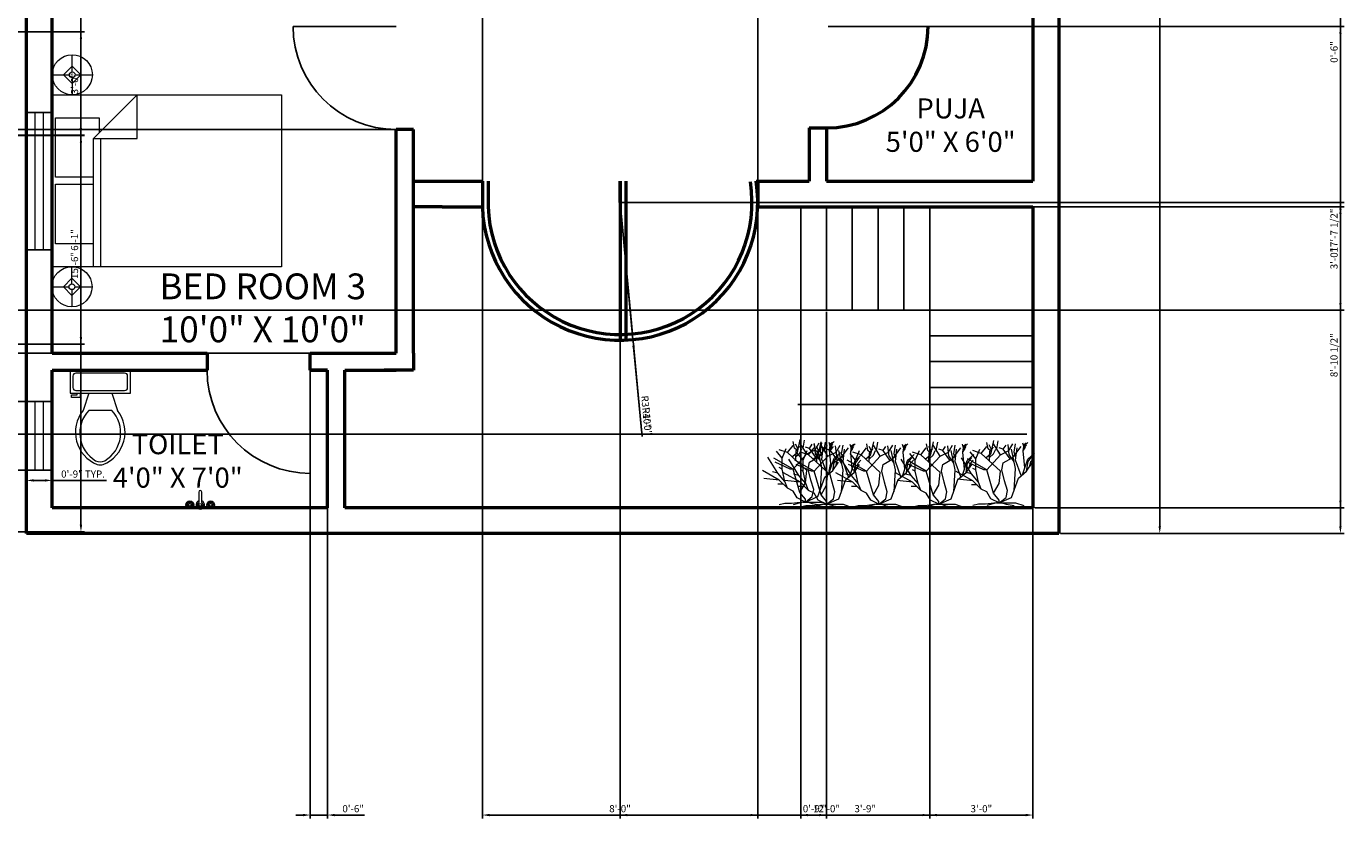
# Model space of a CAD drawing. Units: inches. Extents: x 3688 to 4628, y 1593 to 2337.
# Tile 5 of 7: x 4168 to 4628, y 1596 to 1872. Entities that reach past the tile are written whole.
import ezdxf

# ---------------------------------------------------------------- set-up
doc = ezdxf.new("R2010")
doc.units = ezdxf.units.IN
for name, color, linetype, lineweight in [('A-ANNO-DIMS', 2, 'Continuous', 18), ('A-AREA-IDEN', 7, 'Continuous', 25), ('A-DOOR', 4, 'Continuous', 25), ('A-FLOR-FIXT', 8, 'Continuous', 18), ('A-FLOR-STRS', 3, 'Continuous', 25), ('A-FURN', 8, 'Continuous', 18), ('A-GLAZ', 4, 'Continuous', 25), ('A-WALL', 7, 'Continuous', 50), ('L-PLNT', 3, 'Continuous', 13)]:
    doc.layers.add(name, color=color, linetype=linetype, lineweight=lineweight)
doc.styles.get("Standard").update_dxf_attribs({"font": 'arial.ttf'})
doc.dimstyles.new('ISO-25', dxfattribs={"dimtxt": 2.5, "dimasz": 2.5, "dimexe": 1.25, "dimexo": 0.625, "dimtad": 1, "dimdec": 0, "dimlunit": 3, "dimtxsty": 'Standard', "dimcen": 2.5, "dimadec": 0, "dimazin": 0, "dimtfac": 1, "dimtdec": 0, "dimtmove": 0, "dimatfit": 3, "dimfxl": 1, "dimarcsym": 0})

# ---------------------------------------------------------------- blocks, each defined once
blk = doc.blocks.new('Toilet - top')
for p, q in [((9.5, -6), (9.5, -2)), ((-10, -8.5), (-8, -8.5)), ((-10, -9.5), (-10, -8.5)), ((-8, -8.5), (-8, -8)), ((-7, -8), (-7, -9.5)), ((-4, -8), (-6, -14)), ((4, -8), (6, -14)), ((-7, -9.5), (-10, -9.5)), ((4, -14), (-4, -14))]:
    blk.add_line(p, q)
blk.add_lwpolyline([(10.5, -8), (10.5, 0), (-10.5, 0), (-10.5, -8)], close=True)
for points in [[(-9.5, -2), (-9.5, -6)], [(8.5, -1), (-8.5, -1)], [(-8.5, -7), (8.5, -7)]]:
    blk.add_lwpolyline(points)
for centre, radius, start, end in [((-8.62, -1.88), 0.884, 81.8699, 188.1301), ((8.62, -1.88), 0.884, 351.8699, 98.1301), ((-8.62, -6.12), 0.884, 171.8699, 278.1301), ((8.62, -6.12), 0.884, 261.8699, 8.1301), ((3.52, -21.58), 12.17, 141.4691, 247.9714), ((4.2, -21.82), 11.33, 136.3677, 238.9468), ((-3.52, -21.58), 12.17, 292.0284, 38.5307), ((-4.2, -21.82), 11.33, 301.053, 43.6321), ((0, -27.88), 4, 245.7318, 294.2682), ((0, -29), 4, 254.8605, 285.1395)]:
    blk.add_arc(centre, radius, start, end)
blk = doc.blocks.new('Faucet - Bathroom top')
for p, q in [((-4.107, 0.125), (-4.375, 0.125)), ((-3.75, 0.4788), (-3.75, 0.75)), ((-3.5, 0.482), (-3.5, 0.75)), ((-3.1461, 0.125), (-2.875, 0.125)), ((3.143, 0.125), (2.875, 0.125)), ((3.5, 0.4788), (3.5, 0.75)), ((3.75, 0.482), (3.75, 0.75)), ((4.1039, 0.125), (4.375, 0.125)), ((-4.1039, -0.125), (-4.375, -0.125)), ((-3.75, -0.4821), (-3.75, -0.75)), ((-3.5, -0.4789), (-3.5, -0.75)), ((-3.143, -0.125), (-2.875, -0.125)), ((-0.5, -0.8639), (-0.5, -4.5)), ((0.5, -4.5), (0.5, -0.8631)), ((3.1461, -0.125), (2.875, -0.125)), ((3.5, -0.4821), (3.5, -0.75)), ((3.75, -0.4789), (3.75, -0.75)), ((4.107, -0.125), (4.375, -0.125))]:
    blk.add_line(p, q)
for centre, radius in [((-3.625, 0), 1.375), ((-4.625, 0), 0.2795), ((-3.625, 0), 0.5), ((-3.625, 1), 0.2795), ((-2.625, 0), 0.2795), ((0, 0), 0.5), ((3.625, 0), 1.375), ((2.625, 0), 0.2795), ((3.625, 0), 0.5), ((3.625, 1), 0.2795), ((4.625, 0), 0.2795), ((-3.625, -1), 0.2795), ((3.625, -1), 0.2795)]:
    blk.add_circle(centre, radius)
for centre, radius, start, end in [((-3.625, 0), 1, 105.2407, 164.2093), ((-3.625, 0), 1, 16.44125, 74.07887), ((0, 0), 1.5, 289.6514, 250.3603), ((0, 0), 1, 300.3431, 239.7554), ((3.625, 0), 1, 106.12, 164.0884), ((3.625, 0), 1, 16.23422, 73.90469), ((-3.625, 0), 1, 196.2342, 253.9047), ((-3.625, 0), 1, 286.12, 344.0884), ((0, -4.5), 0.5, 180, 0), ((3.625, 0), 1, 196.4413, 254.0789), ((3.625, 0), 1, 285.2407, 344.2093)]:
    blk.add_arc(centre, radius, start, end)
blk = doc.blocks.new('Bed - Queen')
for p, q in [((0, -80.00003), (0, 0)), ((0, 0), (59.99999, 0)), ((59.99999, 0), (59.99999, -80.00003)), ((7.99999, -1.2), (28.79998, -1.2)), ((7.99999, -14.4), (7.99999, -1.2)), ((28.79998, -1.2), (28.79998, -14.4)), ((31.19999, -1.2), (51.99999, -1.2)), ((31.19999, -14.4), (31.19999, -1.2)), ((51.99999, -1.2), (51.99999, -16.4)), ((0, -14.4), (44.8, -14.4)), ((44.8, -16.8), (0, -16.8)), ((59.99999, -29.6), (44.8, -14.4)), ((44.8, -14.4), (44.8, -29.6)), ((51.99999, -16.4), (46.79936, -16.4)), ((44.8, -29.6), (59.99999, -29.6)), ((59.99999, -80.00003), (0, -80.00003))]:
    blk.add_line(p, q)
blk = doc.blocks.new('Lamp - Table')
for p, q in [((0, 7), (0, 1)), ((-1, 0), (-7, 0)), ((0, 3), (-3, 0)), ((-3, 0), (0, -3)), ((3, 0), (0, 3)), ((0, -3), (3, 0)), ((1, 0), (7, 0)), ((0, -1), (0, -7))]:
    blk.add_line(p, q)
for radius in [7, 1]:
    blk.add_circle((0, 0), radius)
blk = doc.blocks.new('*U12')
for p, q in [((-16.8, 16.32), (-18.72, 18.72)), ((-14.88, 18.24), (-17.76, 19.2)), ((-16.8, 16.32), (-15.36, 19.68)), ((-14.88, 18.24), (-12.96, 20.64)), ((-12.471, 19.775), (-12.898, 22.044)), ((-11.677, 19.071), (-12.471, 19.775)), ((-11.28, 19.619), (-12.104, 21.184)), ((-12.043, 15.628), (-11.921, 18.836)), ((-11.921, 18.836), (-10.64, 20.401)), ((-11.433, 18.289), (-10.457, 22.749)), ((-10.579, 18.054), (-9.846, 19.697)), ((-8.16, 17.76), (-10.56, 21.6)), ((-9.48, 19.775), (-8.992, 22.592)), ((-7.2, 19.68), (-8.64, 20.16)), ((-8.16, 17.76), (-5.28, 19.2)), ((-7.2, 19.68), (-6.24, 21.12)), ((-4.8, 16.32), (-7.2, 19.68)), ((-5.086, 17.741), (-5.513, 21.34)), ((-5.28, 19.2), (-3.84, 21.6)), ((-2.88, 12.96), (-4.32, 19.68)), ((-3.84, 16.8), (-0.96, 20.64)), ((-3.377, 18.602), (-2.888, 21.575)), ((-2.766, 16.802), (-3.377, 18.602)), ((-2.88, 15.84), (-2.4, 20.16)), ((-0.508, 21.888), (-0.081, 20.558)), ((-0.203, 19.149), (0.102, 21.34)), ((0.346, 13.203), (-0.203, 19.149)), ((-0.142, 19.384), (0.59, 20.401)), ((-0.02, 20.01), (0.896, 21.105)), ((0.041, 20.714), (1.384, 22.044)), ((0.102, 21.34), (0.835, 21.888)), ((-18.24, 11.04), (-21.755, 16.655)), ((-12.96, 12.48), (-19.68, 16.32)), ((-13.92, 12.48), (-19.2, 14.88)), ((-16.8, 12.48), (-16.8, 16.32)), ((-8.16, 12), (-14.88, 18.24)), ((-13.325, 16.724), (-11.433, 18.289)), ((-12.96, 12.48), (-8.16, 17.76)), ((-11.982, 16.802), (-10.579, 18.054)), ((-7.68, 12.48), (-7.2, 14.88)), ((-7.2, 14.88), (-3.84, 16.8)), ((-3.377, 15.315), (-5.086, 17.819)), ((-0.96, 10.56), (-2.88, 15.84)), ((0.346, 13.203), (1.323, 16.254)), ((0.96, 12), (1.44, 15.36)), ((0.96, 12), (2.88, 14.88)), ((1.323, 16.254), (3.642, 18.289)), ((1.44, 15.36), (2.88, 17.28)), ((1.92, 13.44), (2.4, 15.36)), ((2.4, 15.36), (3.36, 16.32)), ((-17.76, 8.64), (-23.663, 11.961)), ((-17.76, 8.64), (-23.128, 9.222)), ((-18.24, 11.04), (-20.16, 11.52)), ((-15.84, 8.16), (-18.24, 11.04)), ((-16.8, 12.48), (-17.76, 12.96)), ((-15.84, 8.16), (-16.8, 12.48)), ((-12.96, 12.48), (-13.92, 12.48)), ((-10.56, 4.32), (-12.96, 12.48)), ((-8.64, 7.68), (-8.16, 12)), ((-6.72, 8.64), (-7.68, 12.48)), ((-4.32, 2.88), (-1.92, 9.6)), ((-3.36, 5.28), (-2.88, 12.96)), ((-1.92, 9.6), (0.96, 12)), ((-0.48, 10.8), (0.346, 13.203)), ((-16.32, 7.2), (-18.24, 7.2)), ((-14.88, 5.76), (-17.76, 8.64)), ((-14.88, 5.76), (-15.84, 8.16)), ((-12.96, 4.8), (-14.88, 5.76)), ((-11.52, 2.4), (-12.96, 4.8)), ((-10.56, 4.32), (-8.64, 7.68)), ((-5.76, 5.28), (-6.72, 8.64)), ((-6.24, 2.88), (-5.76, 5.28)), ((-15.84, 0.48), (-17.76, 0)), ((-13.44, 0.48), (-15.84, 0.48)), ((-9.6, 0.96), (-13.44, 0.48)), ((-9.6, 0.96), (-12.96, 0)), ((-8.64, 0.96), (-11.52, 2.4)), ((-8.64, 1.92), (-10.56, 4.32)), ((-9.6, 0.96), (-7.68, 0.96)), ((-8.64, 0.96), (-4.32, 2.88)), ((-8.64, 0.96), (-6.24, 2.88)), ((-8.64, 0.96), (-8.64, 1.92)), ((-8.64, 0.96), (-2.88, 0.96)), ((-7.68, 0.96), (-6.24, 0.48)), ((-6.24, 0.48), (-3.36, 0)), ((-2.88, 0.96), (0, 0))]:
    blk.add_line(p, q)
blk = doc.blocks.new('*D15')
at = {"layer": 'A-ANNO-DIMS', "color": 0, "lineweight": -2, "transparency": 16777216}
for p, q in [((4528.76, 2295.28), (4564.58, 2295.28)), ((4563.33, 2292.78), (4563.33, 1697.78)), ((4528.76, 1695.28), (4564.58, 1695.28))]:
    blk.add_line(p, q, dxfattribs=at)
at = {"layer": 'A-ANNO-DIMS', "color": 0, "transparency": 16777216}
for points in [[(4562.91, 2292.78), (4563.75, 2292.78), (4563.33, 2295.28)], [(4562.91, 1697.78), (4563.75, 1697.78), (4563.33, 1695.28)]]:
    blk.add_solid(points, dxfattribs=at)
at = {"layer": 'Defpoints', "color": 0, "transparency": 16777216}
for p in [(4528.13, 2295.28), (4528.13, 1695.28), (4563.33, 1695.28)]:
    blk.add_point(p, dxfattribs=at)
at = {"layer": 'A-ANNO-DIMS', "color": 0, "transparency": 16777216, "insert": (4561.43, 1995.28), "char_height": 2.5, "attachment_point": 5, "rotation": 90}
blk.add_mtext("50'", dxfattribs=at)
blk = doc.blocks.new('DOOR-900')
blk.add_line((0, 0), (0, 36))
blk.add_arc((0, 0), 36, 0, 90)
blk = doc.blocks.new('WIN-1200')
for p, q in [((0, 48), (0, 0)), ((9, 48), (0, 48)), ((9, 0), (9, 48)), ((0, 0), (9, 0))]:
    blk.add_line(p, q)
blk = doc.blocks.new('WIN-600')
for p, q in [((24, 9), (0, 9)), ((0, 9), (0, 0)), ((24, 0), (24, 9)), ((0, 0), (24, 0))]:
    blk.add_line(p, q)
blk = doc.blocks.new('*D25')
at = {"layer": 'A-ANNO-DIMS', "color": 0, "lineweight": -2, "transparency": 16777216}
for p, q in [((4167.51, 1741.42), (4163.28, 1741.42)), ((4164.53, 1738.92), (4164.53, 1719.92)), ((4167.51, 1717.42), (4163.28, 1717.42)), ((4164.53, 1717.42), (4164.53, 1662.98))]:
    blk.add_line(p, q, dxfattribs=at)
at = {"layer": 'A-ANNO-DIMS', "color": 0, "transparency": 16777216}
for points in [[(4164.12, 1738.92), (4164.95, 1738.92), (4164.53, 1741.42)], [(4164.12, 1719.92), (4164.95, 1719.92), (4164.53, 1717.42)]]:
    blk.add_solid(points, dxfattribs=at)
at = {"layer": 'Defpoints', "color": 0, "transparency": 16777216}
for p in [(4168.13, 1741.42), (4164.53, 1717.42), (4168.13, 1717.42)]:
    blk.add_point(p, dxfattribs=at)
at = {"layer": 'A-ANNO-DIMS', "color": 0, "transparency": 16777216, "insert": (4162.27, 1688.95), "char_height": 2.5, "attachment_point": 5, "rotation": 90}
blk.add_mtext('VENTILATOR V (600) 2\'-0" TYP.', dxfattribs=at)
blk = doc.blocks.new('*D26')
at = {"layer": 'A-ANNO-DIMS', "color": 0, "lineweight": -2, "transparency": 16777216}
for p, q in [((4168.13, 1716.8), (4168.13, 1712.57)), ((4177.13, 1716.8), (4177.13, 1712.57)), ((4170.63, 1713.82), (4174.63, 1713.82)), ((4177.13, 1713.82), (4196.12, 1713.82))]:
    blk.add_line(p, q, dxfattribs=at)
at = {"layer": 'A-ANNO-DIMS', "color": 0, "transparency": 16777216}
for points in [[(4170.63, 1714.24), (4170.63, 1713.41), (4168.13, 1713.82)], [(4174.63, 1714.24), (4174.63, 1713.41), (4177.13, 1713.82)]]:
    blk.add_solid(points, dxfattribs=at)
at = {"layer": 'Defpoints', "color": 0, "transparency": 16777216}
for p in [(4168.13, 1717.42), (4177.13, 1717.42), (4177.13, 1713.82)]:
    blk.add_point(p, dxfattribs=at)
at = {"layer": 'A-ANNO-DIMS', "color": 0, "transparency": 16777216, "insert": (4187.88, 1715.72), "char_height": 2.5, "attachment_point": 5}
blk.add_mtext('0\'-9" TYP.', dxfattribs=at)
blk = doc.blocks.new('*D61')
at = {"layer": 'A-ANNO-DIMS', "color": 0, "lineweight": -2, "transparency": 16777216}
for p, q in [((4090.25, 1881.84), (4188.4, 1881.84)), ((4187.15, 1879.34), (4187.15, 1698.33)), ((4090.03, 1695.83), (4188.4, 1695.83))]:
    blk.add_line(p, q, dxfattribs=at)
at = {"layer": 'A-ANNO-DIMS', "color": 0, "transparency": 16777216}
for points in [[(4186.74, 1879.34), (4187.57, 1879.34), (4187.15, 1881.84)], [(4186.74, 1698.33), (4187.57, 1698.33), (4187.15, 1695.83)]]:
    blk.add_solid(points, dxfattribs=at)
at = {"layer": 'Defpoints', "color": 0, "transparency": 16777216}
for p in [(4089.62, 1881.84), (4089.41, 1695.83), (4187.15, 1695.83)]:
    blk.add_point(p, dxfattribs=at)
at = {"layer": 'A-ANNO-DIMS', "color": 0, "transparency": 16777216, "insert": (4185.25, 1788.83), "char_height": 2.5, "attachment_point": 5, "rotation": 90}
blk.add_mtext('15\'-6"', dxfattribs=at)
blk = doc.blocks.new('*D78')
at = {"layer": 'A-ANNO-DIMS', "color": 0, "lineweight": -2, "transparency": 16777216}
for p, q in [((3973.25, 1870.32), (4188.4, 1870.32)), ((4187.15, 1867.82), (4187.15, 1836.82)), ((3973.25, 1834.32), (4188.4, 1834.32))]:
    blk.add_line(p, q, dxfattribs=at)
at = {"layer": 'A-ANNO-DIMS', "color": 0, "transparency": 16777216}
for points in [[(4186.74, 1867.82), (4187.57, 1867.82), (4187.15, 1870.32)], [(4186.74, 1836.82), (4187.57, 1836.82), (4187.15, 1834.32)]]:
    blk.add_solid(points, dxfattribs=at)
at = {"layer": 'Defpoints', "color": 0, "transparency": 16777216}
for p in [(3972.62, 1870.32), (3972.62, 1834.32), (4187.15, 1834.32)]:
    blk.add_point(p, dxfattribs=at)
at = {"layer": 'A-ANNO-DIMS', "color": 0, "transparency": 16777216, "insert": (4185.25, 1852.32), "char_height": 2.5, "attachment_point": 5, "rotation": 90}
blk.add_mtext('3\'-0"', dxfattribs=at)
blk = doc.blocks.new('*D79')
at = {"layer": 'A-ANNO-DIMS', "color": 0, "lineweight": -2, "transparency": 16777216}
for p, q in [((4044.44, 1834.15), (4188.4, 1834.15)), ((4187.15, 1831.65), (4187.15, 1763.82)), ((4045.25, 1761.32), (4188.4, 1761.32))]:
    blk.add_line(p, q, dxfattribs=at)
at = {"layer": 'A-ANNO-DIMS', "color": 0, "transparency": 16777216}
for points in [[(4186.74, 1831.65), (4187.57, 1831.65), (4187.15, 1834.15)], [(4186.74, 1763.82), (4187.57, 1763.82), (4187.15, 1761.32)]]:
    blk.add_solid(points, dxfattribs=at)
at = {"layer": 'Defpoints', "color": 0, "transparency": 16777216}
for p in [(4043.81, 1834.15), (4044.62, 1761.32), (4187.15, 1761.32)]:
    blk.add_point(p, dxfattribs=at)
at = {"layer": 'A-ANNO-DIMS', "color": 0, "transparency": 16777216, "insert": (4185.25, 1797.73), "char_height": 2.5, "attachment_point": 5, "rotation": 90}
blk.add_mtext('6\'-1"', dxfattribs=at)
blk = doc.blocks.new('*D88')
at = {"layer": 'A-ANNO-DIMS', "color": 0, "lineweight": -2, "transparency": 16777216}
for p, q in [((4528.76, 1906.79), (4627.58, 1906.79)), ((4626.33, 1904.29), (4626.33, 1697.78)), ((4528.76, 1695.28), (4627.58, 1695.28))]:
    blk.add_line(p, q, dxfattribs=at)
at = {"layer": 'A-ANNO-DIMS', "color": 0, "transparency": 16777216}
for points in [[(4625.91, 1904.29), (4626.74, 1904.29), (4626.33, 1906.79)], [(4625.91, 1697.78), (4626.74, 1697.78), (4626.33, 1695.28)]]:
    blk.add_solid(points, dxfattribs=at)
at = {"layer": 'Defpoints', "color": 0, "transparency": 16777216}
for p in [(4528.13, 1906.79), (4528.13, 1695.28), (4626.33, 1695.28)]:
    blk.add_point(p, dxfattribs=at)
at = {"layer": 'A-ANNO-DIMS', "color": 0, "transparency": 16777216, "insert": (4624.41, 1801.03), "char_height": 2.5, "attachment_point": 5, "rotation": 90}
blk.add_mtext('17\'-7 1/2"', dxfattribs=at)
blk = doc.blocks.new('*D100')
at = {"layer": 'A-ANNO-DIMS', "color": 0, "lineweight": -2, "transparency": 16777216}
for p, q in [((4327.13, 1883.66), (4327.13, 1595.79)), ((4423.13, 1883.66), (4423.13, 1595.79)), ((4329.63, 1597.04), (4420.63, 1597.04))]:
    blk.add_line(p, q, dxfattribs=at)
at = {"layer": 'A-ANNO-DIMS', "color": 0, "transparency": 16777216}
for points in [[(4329.63, 1597.45), (4329.63, 1596.62), (4327.13, 1597.04)], [(4420.63, 1597.45), (4420.63, 1596.62), (4423.13, 1597.04)]]:
    blk.add_solid(points, dxfattribs=at)
at = {"layer": 'Defpoints', "color": 0, "transparency": 16777216}
for p in [(4327.13, 1884.28), (4423.13, 1884.28), (4423.13, 1597.04)]:
    blk.add_point(p, dxfattribs=at)
at = {"layer": 'A-ANNO-DIMS', "color": 0, "transparency": 16777216, "insert": (4375.13, 1598.94), "char_height": 2.5, "attachment_point": 5}
blk.add_mtext('8\'-0"', dxfattribs=at)
blk = doc.blocks.new('*D101')
at = {"layer": 'A-ANNO-DIMS', "color": 0, "lineweight": -2, "transparency": 16777216}
for p, q in [((4056.49, 1886.78), (4056.49, 1889.28)), ((4296.51, 1884.28), (4055.24, 1884.28)), ((4056.49, 1884.28), (4056.49, 1878.28)), ((4296.51, 1878.28), (4055.24, 1878.28)), ((4056.49, 1875.78), (4056.49, 1865.39))]:
    blk.add_line(p, q, dxfattribs=at)
at = {"layer": 'A-ANNO-DIMS', "color": 0, "transparency": 16777216}
for points in [[(4056.07, 1886.78), (4056.9, 1886.78), (4056.49, 1884.28)], [(4056.07, 1875.78), (4056.9, 1875.78), (4056.49, 1878.28)]]:
    blk.add_solid(points, dxfattribs=at)
at = {"layer": 'Defpoints', "color": 0, "transparency": 16777216}
for p in [(4297.13, 1884.28), (4056.49, 1878.28), (4297.13, 1878.28)]:
    blk.add_point(p, dxfattribs=at)
at = {"layer": 'A-ANNO-DIMS', "color": 0, "transparency": 16777216, "insert": (4054.58, 1869.34), "char_height": 2.5, "attachment_point": 5, "rotation": 90}
blk.add_mtext('0\'-6"', dxfattribs=at)
blk = doc.blocks.new('*D102')
at = {"layer": 'A-ANNO-DIMS', "color": 0, "lineweight": -2, "transparency": 16777216}
for p, q in [((4296.51, 1836.28), (4055.24, 1836.28)), ((4056.49, 1833.78), (4056.49, 1760.78)), ((4296.51, 1758.28), (4055.24, 1758.28))]:
    blk.add_line(p, q, dxfattribs=at)
at = {"layer": 'A-ANNO-DIMS', "color": 0, "transparency": 16777216}
for points in [[(4056.07, 1833.78), (4056.9, 1833.78), (4056.49, 1836.28)], [(4056.07, 1760.78), (4056.9, 1760.78), (4056.49, 1758.28)]]:
    blk.add_solid(points, dxfattribs=at)
at = {"layer": 'Defpoints', "color": 0, "transparency": 16777216}
for p in [(4297.13, 1836.28), (4056.49, 1758.28), (4297.13, 1758.28)]:
    blk.add_point(p, dxfattribs=at)
at = {"layer": 'A-ANNO-DIMS', "color": 0, "transparency": 16777216, "insert": (4054.58, 1797.28), "char_height": 2.5, "attachment_point": 5, "rotation": 90}
blk.add_mtext('6\'-6"', dxfattribs=at)
blk = doc.blocks.new('*D103')
at = {"layer": 'A-ANNO-DIMS', "color": 0, "lineweight": -2, "transparency": 16777216}
for p, q in [((4626.33, 1880.78), (4626.33, 1883.28)), ((4447.76, 1878.28), (4627.58, 1878.28)), ((4626.33, 1878.28), (4626.33, 1872.28)), ((4447.76, 1872.28), (4627.58, 1872.28)), ((4626.33, 1869.78), (4626.33, 1859.39))]:
    blk.add_line(p, q, dxfattribs=at)
at = {"layer": 'A-ANNO-DIMS', "color": 0, "transparency": 16777216}
for points in [[(4625.91, 1880.78), (4626.74, 1880.78), (4626.33, 1878.28)], [(4625.91, 1869.78), (4626.74, 1869.78), (4626.33, 1872.28)]]:
    blk.add_solid(points, dxfattribs=at)
at = {"layer": 'Defpoints', "color": 0, "transparency": 16777216}
for p in [(4447.13, 1878.28), (4447.13, 1872.28), (4626.33, 1872.28)]:
    blk.add_point(p, dxfattribs=at)
at = {"layer": 'A-ANNO-DIMS', "color": 0, "transparency": 16777216, "insert": (4624.43, 1863.34), "char_height": 2.5, "attachment_point": 5, "rotation": 90}
blk.add_mtext('0\'-6"', dxfattribs=at)
blk = doc.blocks.new('*D104')
at = {"layer": 'A-ANNO-DIMS', "color": 0, "lineweight": -2, "transparency": 16777216}
for p, q in [((4267.13, 1751.66), (4267.13, 1595.79)), ((4273.13, 1751.66), (4273.13, 1595.79)), ((4264.63, 1597.04), (4262.13, 1597.04)), ((4267.13, 1597.04), (4273.13, 1597.04)), ((4275.63, 1597.04), (4286.03, 1597.04))]:
    blk.add_line(p, q, dxfattribs=at)
at = {"layer": 'A-ANNO-DIMS', "color": 0, "transparency": 16777216}
for points in [[(4264.63, 1597.45), (4264.63, 1596.62), (4267.13, 1597.04)], [(4275.63, 1597.45), (4275.63, 1596.62), (4273.13, 1597.04)]]:
    blk.add_solid(points, dxfattribs=at)
at = {"layer": 'Defpoints', "color": 0, "transparency": 16777216}
for p in [(4267.13, 1752.28), (4273.13, 1752.28), (4273.13, 1597.04)]:
    blk.add_point(p, dxfattribs=at)
at = {"layer": 'A-ANNO-DIMS', "color": 0, "transparency": 16777216, "insert": (4282.08, 1598.94), "char_height": 2.5, "attachment_point": 5}
blk.add_mtext('0\'-6"', dxfattribs=at)
blk = doc.blocks.new('*D105')
at = {"layer": 'A-ANNO-DIMS', "color": 0, "lineweight": -2, "transparency": 16777216}
for p, q in [((4375.76, 1810.76), (4627.58, 1810.76)), ((4626.33, 1808.26), (4626.33, 1706.78)), ((4519.76, 1704.28), (4627.58, 1704.28))]:
    blk.add_line(p, q, dxfattribs=at)
at = {"layer": 'A-ANNO-DIMS', "color": 0, "transparency": 16777216}
for points in [[(4625.91, 1808.26), (4626.74, 1808.26), (4626.33, 1810.76)], [(4625.91, 1706.78), (4626.74, 1706.78), (4626.33, 1704.28)]]:
    blk.add_solid(points, dxfattribs=at)
at = {"layer": 'Defpoints', "color": 0, "transparency": 16777216}
for p in [(4375.13, 1810.76), (4519.13, 1704.28), (4626.33, 1704.28)]:
    blk.add_point(p, dxfattribs=at)
at = {"layer": 'A-ANNO-DIMS', "color": 0, "transparency": 16777216, "insert": (4624.41, 1757.52), "char_height": 2.5, "attachment_point": 5, "rotation": 90}
blk.add_mtext('8\'-10 1/2"', dxfattribs=at)
blk = doc.blocks.new('*D106')
at = {"layer": 'A-ANNO-DIMS', "color": 0, "lineweight": -2, "transparency": 16777216}
for p, q in [((4375.13, 1810.13), (4375.13, 1595.79)), ((4519.13, 1808.66), (4519.13, 1595.79)), ((4377.63, 1597.04), (4516.63, 1597.04))]:
    blk.add_line(p, q, dxfattribs=at)
at = {"layer": 'A-ANNO-DIMS', "color": 0, "transparency": 16777216}
for points in [[(4377.63, 1597.45), (4377.63, 1596.62), (4375.13, 1597.04)], [(4516.63, 1597.45), (4516.63, 1596.62), (4519.13, 1597.04)]]:
    blk.add_solid(points, dxfattribs=at)
at = {"layer": 'Defpoints', "color": 0, "transparency": 16777216}
for p in [(4375.13, 1810.76), (4519.13, 1809.28), (4519.13, 1597.04)]:
    blk.add_point(p, dxfattribs=at)
at = {"layer": 'A-ANNO-DIMS', "color": 0, "transparency": 16777216, "insert": (4447.13, 1598.94), "char_height": 2.5, "attachment_point": 5}
blk.add_mtext('12\'-0"', dxfattribs=at)
blk = doc.blocks.new('*D107')
at = {"layer": 'A-ANNO-DIMS', "color": 0, "lineweight": -2, "transparency": 16777216}
for p, q in [((4438.13, 1808.66), (4438.13, 1595.79)), ((4483.13, 1808.66), (4483.13, 1595.79)), ((4440.63, 1597.04), (4480.63, 1597.04))]:
    blk.add_line(p, q, dxfattribs=at)
at = {"layer": 'A-ANNO-DIMS', "color": 0, "transparency": 16777216}
for points in [[(4440.63, 1597.45), (4440.63, 1596.62), (4438.13, 1597.04)], [(4480.63, 1597.45), (4480.63, 1596.62), (4483.13, 1597.04)]]:
    blk.add_solid(points, dxfattribs=at)
at = {"layer": 'Defpoints', "color": 0, "transparency": 16777216}
for p in [(4438.13, 1809.28), (4483.13, 1809.28), (4483.13, 1597.04)]:
    blk.add_point(p, dxfattribs=at)
at = {"layer": 'A-ANNO-DIMS', "color": 0, "transparency": 16777216, "insert": (4460.63, 1598.94), "char_height": 2.5, "attachment_point": 5}
blk.add_mtext('3\'-9"', dxfattribs=at)
blk = doc.blocks.new('*D108')
at = {"layer": 'A-ANNO-DIMS', "color": 0, "lineweight": -2, "transparency": 16777216}
for p, q in [((4483.13, 1808.66), (4483.13, 1595.79)), ((4519.13, 1808.66), (4519.13, 1595.79)), ((4485.63, 1597.04), (4516.63, 1597.04))]:
    blk.add_line(p, q, dxfattribs=at)
at = {"layer": 'A-ANNO-DIMS', "color": 0, "transparency": 16777216}
for points in [[(4485.63, 1597.45), (4485.63, 1596.62), (4483.13, 1597.04)], [(4516.63, 1597.45), (4516.63, 1596.62), (4519.13, 1597.04)]]:
    blk.add_solid(points, dxfattribs=at)
at = {"layer": 'Defpoints', "color": 0, "transparency": 16777216}
for p in [(4483.13, 1809.28), (4519.13, 1809.28), (4519.13, 1597.04)]:
    blk.add_point(p, dxfattribs=at)
at = {"layer": 'A-ANNO-DIMS', "color": 0, "transparency": 16777216, "insert": (4501.13, 1598.94), "char_height": 2.5, "attachment_point": 5}
blk.add_mtext('3\'-0"', dxfattribs=at)
blk = doc.blocks.new('*D109')
at = {"layer": 'A-ANNO-DIMS', "color": 0, "lineweight": -2, "transparency": 16777216}
for p, q in [((4438.13, 1772.66), (4438.13, 1595.79)), ((4447.13, 1772.66), (4447.13, 1595.79)), ((4440.63, 1597.04), (4444.63, 1597.04))]:
    blk.add_line(p, q, dxfattribs=at)
at = {"layer": 'A-ANNO-DIMS', "color": 0, "transparency": 16777216}
for points in [[(4440.63, 1597.45), (4440.63, 1596.62), (4438.13, 1597.04)], [(4444.63, 1597.45), (4444.63, 1596.62), (4447.13, 1597.04)]]:
    blk.add_solid(points, dxfattribs=at)
at = {"layer": 'Defpoints', "color": 0, "transparency": 16777216}
for p in [(4438.13, 1773.28), (4447.13, 1773.28), (4447.13, 1597.04)]:
    blk.add_point(p, dxfattribs=at)
at = {"layer": 'A-ANNO-DIMS', "color": 0, "transparency": 16777216, "insert": (4442.63, 1598.94), "char_height": 2.5, "attachment_point": 5}
blk.add_mtext('0\'-9"', dxfattribs=at)
blk = doc.blocks.new('*D110')
at = {"layer": 'A-ANNO-DIMS', "color": 0, "lineweight": -2, "transparency": 16777216}
for p, q in [((4438.76, 1809.28), (4627.58, 1809.28)), ((4626.33, 1806.78), (4626.33, 1775.78)), ((4438.76, 1773.28), (4627.58, 1773.28))]:
    blk.add_line(p, q, dxfattribs=at)
at = {"layer": 'A-ANNO-DIMS', "color": 0, "transparency": 16777216}
for points in [[(4625.91, 1806.78), (4626.74, 1806.78), (4626.33, 1809.28)], [(4625.91, 1775.78), (4626.74, 1775.78), (4626.33, 1773.28)]]:
    blk.add_solid(points, dxfattribs=at)
at = {"layer": 'Defpoints', "color": 0, "transparency": 16777216}
for p in [(4438.13, 1809.28), (4438.13, 1773.28), (4626.33, 1773.28)]:
    blk.add_point(p, dxfattribs=at)
at = {"layer": 'A-ANNO-DIMS', "color": 0, "transparency": 16777216, "insert": (4624.42, 1791.28), "char_height": 2.5, "attachment_point": 5, "rotation": 90}
blk.add_mtext('3\'-0"', dxfattribs=at)
blk = doc.blocks.new('*D111')
at = {"layer": 'A-ANNO-DIMS', "color": 0, "lineweight": -2, "transparency": 16777216}
for p, q in [((4518.51, 1773.28), (4055.24, 1773.28)), ((4056.49, 1770.78), (4056.49, 1732.46)), ((4516.99, 1729.96), (4055.24, 1729.96))]:
    blk.add_line(p, q, dxfattribs=at)
at = {"layer": 'A-ANNO-DIMS', "color": 0, "transparency": 16777216}
for points in [[(4056.07, 1770.78), (4056.9, 1770.78), (4056.49, 1773.28)], [(4056.07, 1732.46), (4056.9, 1732.46), (4056.49, 1729.96)]]:
    blk.add_solid(points, dxfattribs=at)
at = {"layer": 'Defpoints', "color": 0, "transparency": 16777216}
for p in [(4519.13, 1773.28), (4056.49, 1729.96), (4517.62, 1729.96)]:
    blk.add_point(p, dxfattribs=at)
at = {"layer": 'A-ANNO-DIMS', "color": 0, "transparency": 16777216, "insert": (4054.57, 1751.62), "char_height": 2.5, "attachment_point": 5, "rotation": 90}
blk.add_mtext('3\'-7 1/2"', dxfattribs=at)
blk = doc.blocks.new('*D112')
at = {"layer": 'A-ANNO-DIMS', "color": 0, "lineweight": -2, "transparency": 16777216}
for p, q in [((4375.13, 1810.76), (4379.64, 1762.95)), ((4382.83, 1729.14), (4379.88, 1760.46))]:
    blk.add_line(p, q, dxfattribs=at)
at = {"layer": 'A-ANNO-DIMS', "color": 0, "transparency": 16777216}
blk.add_solid([(4380.29, 1760.5), (4379.46, 1760.42), (4379.64, 1762.95)], dxfattribs=at)
at = {"layer": 'Defpoints', "color": 0, "transparency": 16777216}
for p in [(4375.13, 1810.76), (4379.64, 1762.95)]:
    blk.add_point(p, dxfattribs=at)
at = {"layer": 'A-ANNO-DIMS', "color": 0, "transparency": 16777216, "insert": (4384.24, 1734.44), "char_height": 2.5, "attachment_point": 5, "rotation": 275.3873}
blk.add_mtext('R4\'-0"', dxfattribs=at)
blk = doc.blocks.new('*D113')
at = {"layer": 'A-ANNO-DIMS', "color": 0, "lineweight": -2, "transparency": 16777216}
for p, q in [((4375.13, 1810.76), (4379.45, 1764.94)), ((4382.62, 1731.36), (4379.69, 1762.45))]:
    blk.add_line(p, q, dxfattribs=at)
at = {"layer": 'A-ANNO-DIMS', "color": 0, "transparency": 16777216}
blk.add_solid([(4380.1, 1762.49), (4379.27, 1762.41), (4379.45, 1764.94)], dxfattribs=at)
at = {"layer": 'Defpoints', "color": 0, "transparency": 16777216}
for p in [(4375.13, 1810.76), (4379.45, 1764.94)]:
    blk.add_point(p, dxfattribs=at)
at = {"layer": 'A-ANNO-DIMS', "color": 0, "transparency": 16777216, "insert": (4383.94, 1737.63), "char_height": 2.5, "attachment_point": 5, "rotation": 275.387}
blk.add_mtext('R3\'-10"', dxfattribs=at)

msp = doc.modelspace()

# ---------------------------------------------------------------- linework, layer by layer
at = {"layer": 'A-FLOR-STRS'}
for p, q in [((4438.13, 1809.28), (4438.13, 1773.28)), ((4447.13, 1809.28), (4447.13, 1773.28)), ((4456.13, 1809.28), (4456.13, 1773.28)), ((4465.13, 1809.28), (4465.13, 1773.28)), ((4474.13, 1809.28), (4474.13, 1773.28)), ((4483.13, 1809.28), (4483.13, 1740.28)), ((4438.13, 1773.28), (4519.13, 1773.28)), ((4483.13, 1764.28), (4519.13, 1764.28)), ((4483.13, 1755.28), (4519.13, 1755.28)), ((4483.13, 1746.28), (4519.13, 1746.28)), ((4483.13, 1740.28), (4437.11, 1740.28)), ((4519.13, 1740.28), (4483.13, 1740.28))]:
    msp.add_line(p, q, dxfattribs=at)
at = {"layer": 'A-FURN'}
for p, q in [((4171.13, 1842.28), (4171.13, 1794.28)), ((4174.13, 1794.28), (4174.13, 1842.28)), ((4171.13, 1741.42), (4171.13, 1717.42)), ((4174.13, 1717.42), (4174.13, 1741.42))]:
    msp.add_line(p, q, dxfattribs=at)
at = {"layer": 'A-WALL'}
for p, q in [((4168.13, 1695.28), (4168.13, 2295.28)), ((4528.13, 2295.28), (4528.13, 1695.28)), ((4177.13, 1758.28), (4177.13, 1878.28)), ((4519.13, 1878.28), (4519.13, 1818.28)), ((4297.13, 1758.28), (4297.13, 1836.28)), ((4303.13, 1836.28), (4297.13, 1836.28)), ((4303.13, 1818.28), (4303.13, 1836.28)), ((4303.13, 1758.28), (4303.13, 1836.28)), ((4441.13, 1836.84), (4447.13, 1836.84)), ((4441.13, 1836.84), (4441.13, 1818.28)), ((4447.13, 1836.84), (4447.13, 1818.28)), ((4303.13, 1818.28), (4327.13, 1818.28)), ((4303.13, 1818.28), (4313.13, 1818.28)), ((4327.13, 1818.28), (4327.13, 1809.28)), ((4329.13, 1818.28), (4329.13, 1809.28)), ((4375.13, 1810.76), (4375.13, 1818.28)), ((4375.13, 1818.28), (4375.13, 1762.74)), ((4377.13, 1818.28), (4377.13, 1762.74)), ((4422.56, 1818.28), (4441.13, 1818.28)), ((4423.13, 1818.28), (4423.13, 1809.28)), ((4447.13, 1818.28), (4519.13, 1818.28)), ((4313.13, 1809.28), (4303.13, 1809.28)), ((4313.13, 1809.28), (4327.13, 1809.28)), ((4423.13, 1809.28), (4519.13, 1809.28)), ((4519.13, 1809.28), (4519.13, 1704.28)), ((4177.13, 1758.28), (4231.13, 1758.28)), ((4231.13, 1758.28), (4231.13, 1752.28)), ((4267.13, 1758.28), (4297.13, 1758.28)), ((4267.13, 1752.28), (4267.13, 1758.28)), ((4303.13, 1758.28), (4303.13, 1752.29)), ((4177.13, 1752.28), (4231.13, 1752.28)), ((4177.13, 1749.28), (4177.13, 1752.28)), ((4177.13, 1704.28), (4177.13, 1749.28)), ((4267.13, 1752.28), (4273.13, 1752.28)), ((4273.13, 1752.28), (4267.13, 1752.28)), ((4273.13, 1749.28), (4273.13, 1752.28)), ((4273.13, 1704.28), (4273.13, 1749.28)), ((4279.13, 1749.28), (4279.13, 1752.28)), ((4279.13, 1752.28), (4297.13, 1752.28)), ((4279.13, 1704.28), (4279.13, 1749.28)), ((4303.13, 1752.29), (4292.92, 1752.28)), ((4273.13, 1704.28), (4177.13, 1704.28)), ((4519.13, 1704.28), (4279.13, 1704.28)), ((4528.13, 1695.28), (4168.13, 1695.28))]:
    msp.add_line(p, q, dxfattribs=at)
for centre, radius, start, end in [((4447.13, 1872.28), 35.44, 270, 0), ((4375.13, 1810.76), 48.02, 181.7618, 9.0135), ((4375.13, 1810.76), 46.02, 181.7618, 9.0135)]:
    msp.add_arc(centre, radius, start, end, dxfattribs=at)

# ---------------------------------------------------------------- block references
at = {"layer": 'A-DOOR', "extrusion": (0, 0, -1), "zscale": -1, "rotation": 270}
msp.add_blockref('DOOR-900', (-4297.13, 1872.28), dxfattribs=at)
at = {"layer": 'A-DOOR', "rotation": 180}
msp.add_blockref('DOOR-900', (4267.13, 1752.28), dxfattribs=at)
at = {"layer": 'A-FLOR-FIXT'}
msp.add_blockref('Toilet - top', (4193.88, 1752.23), dxfattribs=at)
at = {"layer": 'A-FLOR-FIXT', "rotation": 180}
msp.add_blockref('Faucet - Bathroom top', (4228.76, 1705.28), dxfattribs=at)
at = {"layer": 'A-FURN', "rotation": 90}
for name, p in [('Lamp - Table', (4184.13, 1855.4)), ('Bed - Queen', (4177.13, 1788.4)), ('Lamp - Table', (4184.03, 1781.4))]:
    msp.add_blockref(name, p, dxfattribs=at)
at = {"layer": 'A-GLAZ'}
msp.add_blockref('WIN-1200', (4168.13, 1794.28), dxfattribs=at)
at = {"layer": 'A-GLAZ', "rotation": 270.0000000000038}
msp.add_blockref('WIN-600', (4168.13, 1741.42), dxfattribs=at)
at = {"layer": 'L-PLNT'}
for p in [(4448.42, 1705.32), (4455.77, 1704.53), (4474.05, 1704.53), (4494.89, 1704.53), (4515.96, 1705.03)]:
    msp.add_blockref('*U12', p, dxfattribs=at)

# ---------------------------------------------------------------- texts
at = {"layer": 'A-AREA-IDEN', "attachment_point": 1}
for s, width, insert, char_height in [('\\pxqc;PUJA\\P5\'0" X 6\'0"', 61.3205, (4459.77, 1847.16), 7), ('\\pxqc;BED ROOM 3\\P10\'0" X 10\'0"', 105.0766, (4198.01, 1786.05), 9), ('\\pxqc;TOILET \\P4\'0" X 7\'0"', 61.3205, (4190.25, 1729.97), 7)]:
    msp.add_mtext_dynamic_manual_height_columns(s, width=width, gutter_width=12.5, heights=[0], dxfattribs=dict(at, insert=insert, char_height=char_height))

# ---------------------------------------------------------------- dimensions: what is measured, and where the dimension line sits
at = {"layer": 'A-ANNO-DIMS'}
for base, p1, p2, override, picture, middle in [((4563.33, 1695.28), (4528.13, 2295.28), (4528.13, 1695.28), {"dimclrd": 0, "dimclre": 0, "dimclrt": 0}, '*D15', (4561.43, 1995.28)), ((4626.33, 1695.28), (4528.13, 1906.79), (4528.13, 1695.28), {"dimdec": 1, "dimlfac": 1, "dimrnd": 0, "dimzin": 1, "dimdsep": 46, "dimlunit": 4, "dimfrac": 2}, '*D88', (4624.41, 1801.03)), ((4056.49, 1878.28), (4297.13, 1884.28), (4297.13, 1878.28), {"dimdec": 1, "dimlfac": 1, "dimrnd": 0, "dimzin": 1, "dimdsep": 46, "dimlunit": 4, "dimfrac": 2}, '*D101', (4054.58, 1869.34)), ((4187.15, 1695.83), (4089.62, 1881.84), (4089.41, 1695.83), {"dimdec": 1, "dimlfac": 1, "dimrnd": 0, "dimzin": 1, "dimdsep": 46, "dimlunit": 4, "dimfrac": 2}, '*D61', (4185.25, 1788.83)), ((4626.33, 1872.28), (4447.13, 1878.28), (4447.13, 1872.28), {"dimdec": 1, "dimlfac": 1, "dimrnd": 0, "dimzin": 1, "dimdsep": 46, "dimlunit": 4, "dimfrac": 2}, '*D103', (4624.43, 1863.34)), ((4187.15, 1834.32), (3972.62, 1870.32), (3972.62, 1834.32), {"dimdec": 1, "dimlfac": 1, "dimrnd": 0, "dimzin": 1, "dimdsep": 46, "dimlunit": 4, "dimfrac": 2}, '*D78', (4185.25, 1852.32)), ((4056.49, 1758.28), (4297.13, 1836.28), (4297.13, 1758.28), {"dimdec": 1, "dimlfac": 1, "dimrnd": 0, "dimzin": 1, "dimdsep": 46, "dimlunit": 4, "dimfrac": 2}, '*D102', (4054.58, 1797.28)), ((4187.15, 1761.32), (4043.81, 1834.15), (4044.62, 1761.32), {"dimdec": 1, "dimlfac": 1, "dimrnd": 0, "dimzin": 1, "dimdsep": 46, "dimlunit": 4, "dimfrac": 2}, '*D79', (4185.25, 1797.73)), ((4626.33, 1704.28), (4375.13, 1810.76), (4519.13, 1704.28), {"dimdec": 1, "dimlfac": 1, "dimrnd": 0, "dimzin": 1, "dimdsep": 46, "dimlunit": 4, "dimfrac": 2}, '*D105', (4624.41, 1757.52)), ((4626.33, 1773.28), (4438.13, 1809.28), (4438.13, 1773.28), {"dimdec": 1, "dimlfac": 1, "dimrnd": 0, "dimzin": 1, "dimdsep": 46, "dimlunit": 4, "dimfrac": 2}, '*D110', (4624.42, 1791.28)), ((4056.49, 1729.96), (4519.13, 1773.28), (4517.62, 1729.96), {"dimdec": 1, "dimlfac": 1, "dimrnd": 0, "dimzin": 1, "dimdsep": 46, "dimlunit": 4, "dimfrac": 2}, '*D111', (4054.57, 1751.62))]:
    dim = msp.add_linear_dim(base=base, p1=p1, p2=p2, angle=90, dimstyle='ISO-25', override=override, dxfattribs=at)
    dim.commit()
    dim.dimension.update_dxf_attribs({"geometry": picture, "text_midpoint": middle})
for base, p1, p2, picture, middle in [((4423.13, 1597.04), (4327.13, 1884.28), (4423.13, 1884.28), '*D100', (4375.13, 1598.94)), ((4519.13, 1597.04), (4375.13, 1810.76), (4519.13, 1809.28), '*D106', (4447.13, 1598.94)), ((4483.13, 1597.04), (4438.13, 1809.28), (4483.13, 1809.28), '*D107', (4460.63, 1598.94)), ((4519.13, 1597.04), (4483.13, 1809.28), (4519.13, 1809.28), '*D108', (4501.13, 1598.94)), ((4447.13, 1597.04), (4438.13, 1773.28), (4447.13, 1773.28), '*D109', (4442.63, 1598.94)), ((4273.13, 1597.04), (4267.13, 1752.28), (4273.13, 1752.28), '*D104', (4282.08, 1598.94))]:
    dim = msp.add_linear_dim(base=base, p1=p1, p2=p2, dimstyle='ISO-25', override={"dimdec": 1, "dimlfac": 1, "dimrnd": 0, "dimzin": 1, "dimdsep": 46, "dimlunit": 4, "dimfrac": 2}, dxfattribs=at)
    dim.commit()
    dim.dimension.update_dxf_attribs({"geometry": picture, "text_midpoint": middle})
for mpoint, picture, middle in [((4379.64, 1762.95), '*D112', (4382.35, 1734.26)), ((4379.45, 1764.94), '*D113', (4382.05, 1737.45))]:
    dim = msp.add_radius_dim(center=(4375.13, 1810.76), mpoint=mpoint, dimstyle='ISO-25', override={"dimdec": 1, "dimlfac": 1, "dimrnd": 0, "dimzin": 1, "dimdsep": 46, "dimlunit": 4, "dimfrac": 2}, dxfattribs=at)
    dim.commit()
    dim.dimension.update_dxf_attribs({"geometry": picture, "text_midpoint": middle, "dimtype": 164})
for base, p1, p2, angle, text, picture, middle in [((4164.53, 1717.42), (4168.13, 1741.42), (4168.13, 1717.42), 270, 'VENTILATOR V (600) <> TYP.', '*D25', (4162.27, 1688.95)), ((4177.13, 1713.82), (4168.13, 1717.42), (4177.13, 1717.42), 0, '<> TYP.', '*D26', (4187.88, 1715.72))]:
    dim = msp.add_linear_dim(base=base, p1=p1, p2=p2, angle=angle, text=text, dimstyle='ISO-25', override={"dimdec": 1, "dimrnd": 0, "dimzin": 1, "dimlunit": 4, "dimfrac": 2}, dxfattribs=at)
    dim.commit()
    dim.dimension.update_dxf_attribs({"geometry": picture, "text_midpoint": middle})

doc.saveas('drawing.dxf')
